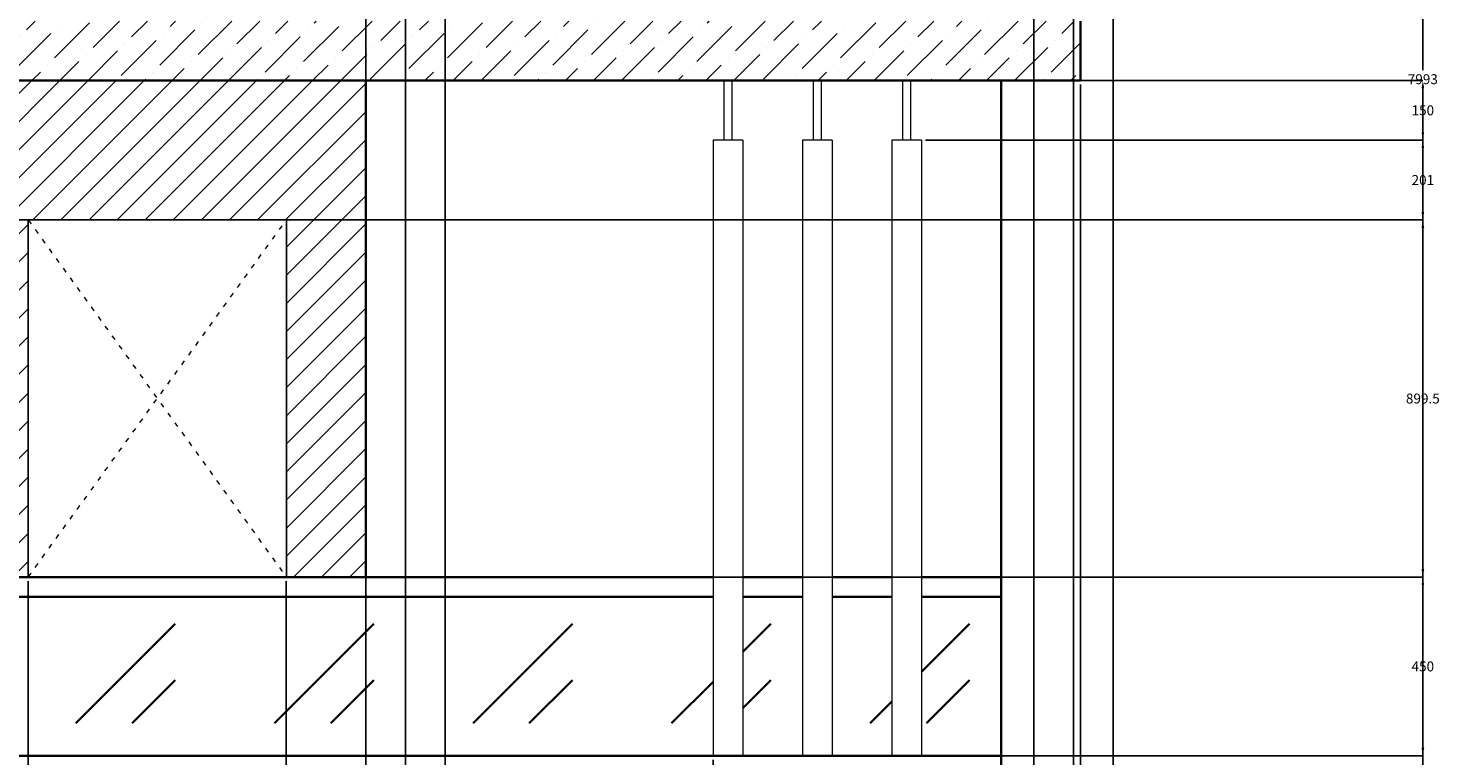
# Model space of a CAD drawing. Units: millimetres. Extents: x -692 to 9639, y -141 to 10345.
# Tile 10 of 19: x 6042 to 9596, y 3148 to 4981. Entities that reach past the tile are written whole.
import ezdxf

# ---------------------------------------------------------------- set-up
doc = ezdxf.new("R2010")
doc.units = ezdxf.units.MM
doc.header["$MEASUREMENT"] = 0
doc.linetypes.add('ACAD_ISO03W100', pattern=[30, 12, -18])
for name, color, linetype, lineweight in [('A-ANNO-DIMS', 2, 'Continuous', 18), ('A-DOOR', 3, 'Continuous', 25), ('A-DOOR-SWNG', 3, 'ACAD_ISO03W100', 18), ('A-ELEV', 7, 'Continuous', 35), ('A-ELEV-DECO', 4, 'Continuous', 18), ('A-ELEV-PATT', 8, 'Continuous', 13)]:
    doc.layers.add(name, color=color, linetype=linetype, lineweight=lineweight)
doc.styles.get("Standard").update_dxf_attribs({"font": 'arial.ttf'})
doc.dimstyles.get("Standard").update_dxf_attribs({"dimtxt": 25, "dimasz": 20, "dimexe": 0.18, "dimexo": 10, "dimgap": 10, "dimtad": 0, "dimtih": 1, "dimtoh": 1, "dimdec": 0, "dimzin": 0, "dimdsep": 46, "dimtxsty": 'Standard', "dimcen": 10, "dimadec": 0, "dimazin": 0, "dimtfac": 1, "dimtdec": 0, "dimtofl": 0, "dimtmove": 0, "dimatfit": 3, "dimfxl": 1, "dimtolj": 1, "dimtzin": 0, "dimarcsym": 0})

# ---------------------------------------------------------------- blocks, each defined once
blk = doc.blocks.new('*D7')
at = {"layer": 'A-ANNO-DIMS', "color": 0, "lineweight": -2, "transparency": 16777216}
for p, q in [((8481.5, 9848.8), (-649.1, 9848.8)), ((-648.9, 9828.8), (-648.9, 5124.9)), ((-648.9, 375.6), (-648.9, 5079.4)), ((2463.7, 355.6), (-649.1, 355.6))]:
    blk.add_line(p, q, dxfattribs=at)
at = {"layer": 'A-ANNO-DIMS', "color": 0, "lineweight": -3, "transparency": 16777216}
for points in [[(-652.2, 9828.8), (-645.6, 9828.8), (-648.9, 9848.8)], [(-652.2, 375.6), (-645.6, 375.6), (-648.9, 355.6)]]:
    blk.add_solid(points, dxfattribs=at)
at = {"layer": 'Defpoints', "color": 0, "lineweight": -3, "transparency": 16777216}
for p in [(-648.9, 9848.8), (8491.5, 9848.8), (2473.7, 355.6)]:
    blk.add_point(p, dxfattribs=at)
at = {"layer": 'A-ANNO-DIMS', "color": 0, "transparency": 16777216, "insert": (-648.9, 5102.2), "char_height": 25, "attachment_point": 5}
blk.add_mtext('\\A1;9493', dxfattribs=at)
blk = doc.blocks.new('*D9')
at = {"layer": 'A-ANNO-DIMS', "color": 0, "lineweight": -2, "transparency": 16777216}
for p, q in [((8501.5, 8848.8), (9553.9, 8848.8)), ((9553.7, 8828.8), (9553.7, 4874.9)), ((9553.7, 875.6), (9553.7, 4829.4)), ((9083.7, 855.6), (9553.9, 855.6))]:
    blk.add_line(p, q, dxfattribs=at)
at = {"layer": 'A-ANNO-DIMS', "color": 0, "lineweight": -3, "transparency": 16777216}
for points in [[(9550.4, 8828.8), (9557.1, 8828.8), (9553.7, 8848.8)], [(9550.4, 875.6), (9557.1, 875.6), (9553.7, 855.6)]]:
    blk.add_solid(points, dxfattribs=at)
at = {"layer": 'Defpoints', "color": 0, "lineweight": -3, "transparency": 16777216}
for p in [(8491.5, 8848.8), (9553.7, 8848.8), (9073.7, 855.6)]:
    blk.add_point(p, dxfattribs=at)
at = {"layer": 'A-ANNO-DIMS', "color": 0, "transparency": 16777216, "insert": (9553.7, 4852.2), "char_height": 25, "attachment_point": 5}
blk.add_mtext('\\A1;7993', dxfattribs=at)
blk = doc.blocks.new('*D32')
at = {"layer": 'A-ANNO-DIMS', "color": 0, "lineweight": -2, "transparency": 16777216}
for p, q in [((6871.7, 10328.8), (6851.7, 10328.8)), ((6891.7, 1865.6), (6891.7, 10329)), ((6991.7, 1765.6), (6991.7, 10329)), ((7011.7, 10328.8), (7031.7, 10328.8))]:
    blk.add_line(p, q, dxfattribs=at)
at = {"layer": 'A-ANNO-DIMS', "color": 0, "lineweight": -3, "transparency": 16777216}
for points in [[(6871.7, 10332.1), (6871.7, 10325.4), (6891.7, 10328.8)], [(7011.7, 10332.1), (7011.7, 10325.4), (6991.7, 10328.8)]]:
    blk.add_solid(points, dxfattribs=at)
at = {"layer": 'Defpoints', "color": 0, "lineweight": -3, "transparency": 16777216}
for p in [(6991.7, 10328.8), (6891.7, 1855.6), (6991.7, 1755.6)]:
    blk.add_point(p, dxfattribs=at)
at = {"layer": 'A-ANNO-DIMS', "color": 0, "transparency": 16777216, "insert": (6941.7, 10328.8), "char_height": 25, "attachment_point": 5}
blk.add_mtext('\\A1;100', dxfattribs=at)
blk = doc.blocks.new('*D33')
at = {"layer": 'A-ANNO-DIMS', "color": 0, "lineweight": -2, "transparency": 16777216}
for p, q in [((6971.7, 10328.8), (6951.7, 10328.8)), ((6991.7, 1765.6), (6991.7, 10329)), ((7091.7, 1665.6), (7091.7, 10329)), ((7111.7, 10328.8), (7131.7, 10328.8))]:
    blk.add_line(p, q, dxfattribs=at)
at = {"layer": 'A-ANNO-DIMS', "color": 0, "lineweight": -3, "transparency": 16777216}
for points in [[(6971.7, 10332.1), (6971.7, 10325.4), (6991.7, 10328.8)], [(7111.7, 10332.1), (7111.7, 10325.4), (7091.7, 10328.8)]]:
    blk.add_solid(points, dxfattribs=at)
at = {"layer": 'Defpoints', "color": 0, "lineweight": -3, "transparency": 16777216}
for p in [(7091.7, 10328.8), (6991.7, 1755.6), (7091.7, 1655.6)]:
    blk.add_point(p, dxfattribs=at)
at = {"layer": 'A-ANNO-DIMS', "color": 0, "transparency": 16777216, "insert": (7041.7, 10328.8), "char_height": 25, "attachment_point": 5}
blk.add_mtext('\\A1;100', dxfattribs=at)
blk = doc.blocks.new('*D34')
at = {"layer": 'A-ANNO-DIMS', "color": 0, "lineweight": -2, "transparency": 16777216}
for p, q in [((7091.7, 1665.6), (7091.7, 10329)), ((7111.7, 10328.8), (7786.7, 10328.8)), ((8553.7, 10328.8), (7878.8, 10328.8)), ((8573.7, 1665.6), (8573.7, 10329))]:
    blk.add_line(p, q, dxfattribs=at)
at = {"layer": 'A-ANNO-DIMS', "color": 0, "lineweight": -3, "transparency": 16777216}
for points in [[(7111.7, 10332.1), (7111.7, 10325.4), (7091.7, 10328.8)], [(8553.7, 10332.1), (8553.7, 10325.4), (8573.7, 10328.8)]]:
    blk.add_solid(points, dxfattribs=at)
at = {"layer": 'Defpoints', "color": 0, "lineweight": -3, "transparency": 16777216}
for p in [(8573.7, 10328.8), (7091.7, 1655.6), (8573.7, 1655.6)]:
    blk.add_point(p, dxfattribs=at)
at = {"layer": 'A-ANNO-DIMS', "color": 0, "transparency": 16777216, "insert": (7832.7, 10328.8), "char_height": 25, "attachment_point": 5}
blk.add_mtext('\\A1;1482', dxfattribs=at)
blk = doc.blocks.new('*D35')
at = {"layer": 'A-ANNO-DIMS', "color": 0, "lineweight": -2, "transparency": 16777216}
for p, q in [((8553.7, 10328.8), (8533.7, 10328.8)), ((8573.7, 1665.6), (8573.7, 10329)), ((8673.7, 1765.6), (8673.7, 10329)), ((8693.7, 10328.8), (8713.7, 10328.8))]:
    blk.add_line(p, q, dxfattribs=at)
at = {"layer": 'A-ANNO-DIMS', "color": 0, "lineweight": -3, "transparency": 16777216}
for points in [[(8553.7, 10332.1), (8553.7, 10325.4), (8573.7, 10328.8)], [(8693.7, 10332.1), (8693.7, 10325.4), (8673.7, 10328.8)]]:
    blk.add_solid(points, dxfattribs=at)
at = {"layer": 'Defpoints', "color": 0, "lineweight": -3, "transparency": 16777216}
for p in [(8673.7, 10328.8), (8673.7, 1755.6), (8573.7, 1655.6)]:
    blk.add_point(p, dxfattribs=at)
at = {"layer": 'A-ANNO-DIMS', "color": 0, "transparency": 16777216, "insert": (8623.7, 10328.8), "char_height": 25, "attachment_point": 5}
blk.add_mtext('\\A1;100', dxfattribs=at)
blk = doc.blocks.new('*D36')
at = {"layer": 'A-ANNO-DIMS', "color": 0, "lineweight": -2, "transparency": 16777216}
for p, q in [((8653.7, 10328.8), (8633.7, 10328.8)), ((8673.7, 1765.6), (8673.7, 10329)), ((8773.7, 1865.6), (8773.7, 10329)), ((8793.7, 10328.8), (8813.7, 10328.8))]:
    blk.add_line(p, q, dxfattribs=at)
at = {"layer": 'A-ANNO-DIMS', "color": 0, "lineweight": -3, "transparency": 16777216}
for points in [[(8653.7, 10332.1), (8653.7, 10325.4), (8673.7, 10328.8)], [(8793.7, 10332.1), (8793.7, 10325.4), (8773.7, 10328.8)]]:
    blk.add_solid(points, dxfattribs=at)
at = {"layer": 'Defpoints', "color": 0, "lineweight": -3, "transparency": 16777216}
for p in [(8773.7, 10328.8), (8773.7, 1855.6), (8673.7, 1755.6)]:
    blk.add_point(p, dxfattribs=at)
at = {"layer": 'A-ANNO-DIMS', "color": 0, "transparency": 16777216, "insert": (8723.7, 10328.8), "char_height": 25, "attachment_point": 5}
blk.add_mtext('\\A1;100', dxfattribs=at)
blk = doc.blocks.new('*D42')
at = {"layer": 'A-ANNO-DIMS', "color": 0, "lineweight": -2, "transparency": 16777216}
for p, q in [((6041.7, 3588.3), (6041.7, -124.6)), ((6691.7, 3588.3), (6691.7, -124.6)), ((6061.7, -124.4), (6329.1, -124.4)), ((6671.7, -124.4), (6404.4, -124.4))]:
    blk.add_line(p, q, dxfattribs=at)
at = {"layer": 'A-ANNO-DIMS', "color": 0, "lineweight": -3, "transparency": 16777216}
for points in [[(6061.7, -121.1), (6061.7, -127.8), (6041.7, -124.4)], [(6671.7, -121.1), (6671.7, -127.8), (6691.7, -124.4)]]:
    blk.add_solid(points, dxfattribs=at)
at = {"layer": 'Defpoints', "color": 0, "lineweight": -3, "transparency": 16777216}
for p in [(6041.7, 3598.3), (6691.7, 3598.3), (6691.7, -124.4)]:
    blk.add_point(p, dxfattribs=at)
at = {"layer": 'A-ANNO-DIMS', "color": 0, "transparency": 16777216, "insert": (6366.7, -124.4), "char_height": 25, "attachment_point": 5}
blk.add_mtext('\\A1;650', dxfattribs=at)
blk = doc.blocks.new('*D43')
at = {"layer": 'A-ANNO-DIMS', "color": 0, "lineweight": -2, "transparency": 16777216}
for p, q in [((6691.7, 3588.3), (6691.7, -124.6)), ((6891.7, 3588.3), (6891.7, -124.6)), ((6711.7, -124.4), (6754, -124.4)), ((6871.7, -124.4), (6829.5, -124.4))]:
    blk.add_line(p, q, dxfattribs=at)
at = {"layer": 'A-ANNO-DIMS', "color": 0, "lineweight": -3, "transparency": 16777216}
for points in [[(6711.7, -121.1), (6711.7, -127.8), (6691.7, -124.4)], [(6871.7, -121.1), (6871.7, -127.8), (6891.7, -124.4)]]:
    blk.add_solid(points, dxfattribs=at)
at = {"layer": 'Defpoints', "color": 0, "lineweight": -3, "transparency": 16777216}
for p in [(6691.7, 3598.3), (6891.7, 3598.3), (6891.7, -124.4)]:
    blk.add_point(p, dxfattribs=at)
at = {"layer": 'A-ANNO-DIMS', "color": 0, "transparency": 16777216, "insert": (6791.7, -124.4), "char_height": 25, "attachment_point": 5}
blk.add_mtext('\\A1;200', dxfattribs=at)
blk = doc.blocks.new('*D44')
at = {"layer": 'A-ANNO-DIMS', "color": 0, "lineweight": -2, "transparency": 16777216}
for p, q in [((6891.7, 3588.3), (6891.7, -124.6)), ((7766.5, 3138.3), (7766.5, -124.6)), ((6911.7, -124.4), (7276.9, -124.4)), ((7746.5, -124.4), (7381.4, -124.4))]:
    blk.add_line(p, q, dxfattribs=at)
at = {"layer": 'A-ANNO-DIMS', "color": 0, "lineweight": -3, "transparency": 16777216}
for points in [[(6911.7, -121.1), (6911.7, -127.8), (6891.7, -124.4)], [(7746.5, -121.1), (7746.5, -127.8), (7766.5, -124.4)]]:
    blk.add_solid(points, dxfattribs=at)
at = {"layer": 'Defpoints', "color": 0, "lineweight": -3, "transparency": 16777216}
for p in [(6891.7, 3598.3), (7766.5, 3148.3), (7766.5, -124.4)]:
    blk.add_point(p, dxfattribs=at)
at = {"layer": 'A-ANNO-DIMS', "color": 0, "transparency": 16777216, "insert": (7329.1, -124.4), "char_height": 25, "attachment_point": 5}
blk.add_mtext('\\A1;874.8', dxfattribs=at)
blk = doc.blocks.new('*D51')
at = {"layer": 'A-ANNO-DIMS', "color": 0, "lineweight": -2, "transparency": 16777216}
for p, q in [((8691.5, 4838.8), (8691.5, -124.6)), ((8491.5, 3138.3), (8491.5, -124.6)), ((8511.5, -124.4), (8553.8, -124.4)), ((8671.5, -124.4), (8629.3, -124.4))]:
    blk.add_line(p, q, dxfattribs=at)
at = {"layer": 'A-ANNO-DIMS', "color": 0, "lineweight": -3, "transparency": 16777216}
for points in [[(8511.5, -121.1), (8511.5, -127.8), (8491.5, -124.4)], [(8671.5, -121.1), (8671.5, -127.8), (8691.5, -124.4)]]:
    blk.add_solid(points, dxfattribs=at)
at = {"layer": 'Defpoints', "color": 0, "lineweight": -3, "transparency": 16777216}
for p in [(8691.5, 4848.8), (8491.5, 3148.3), (8691.5, -124.4)]:
    blk.add_point(p, dxfattribs=at)
at = {"layer": 'A-ANNO-DIMS', "color": 0, "transparency": 16777216, "insert": (8591.5, -124.4), "char_height": 25, "attachment_point": 5}
blk.add_mtext('\\A1;200', dxfattribs=at)
blk = doc.blocks.new('*D71')
at = {"layer": 'A-ANNO-DIMS', "color": 0, "lineweight": -2, "transparency": 16777216}
for p, q in [((5201.5, 3598.3), (9553.9, 3598.3)), ((9553.7, 3578.3), (9553.7, 3396)), ((9553.7, 3168.3), (9553.7, 3350.5)), ((5101.5, 3148.3), (9553.9, 3148.3))]:
    blk.add_line(p, q, dxfattribs=at)
at = {"layer": 'A-ANNO-DIMS', "color": 0, "lineweight": -3, "transparency": 16777216}
for points in [[(9550.4, 3578.3), (9557.1, 3578.3), (9553.7, 3598.3)], [(9550.4, 3168.3), (9557.1, 3168.3), (9553.7, 3148.3)]]:
    blk.add_solid(points, dxfattribs=at)
at = {"layer": 'Defpoints', "color": 0, "lineweight": -3, "transparency": 16777216}
for p in [(5191.5, 3598.3), (9553.7, 3598.3), (5091.5, 3148.3)]:
    blk.add_point(p, dxfattribs=at)
at = {"layer": 'A-ANNO-DIMS', "color": 0, "transparency": 16777216, "insert": (9553.7, 3373.3), "char_height": 25, "attachment_point": 5}
blk.add_mtext('\\A1;450', dxfattribs=at)
blk = doc.blocks.new('*D72')
at = {"layer": 'A-ANNO-DIMS', "color": 0, "lineweight": -2, "transparency": 16777216}
for p, q in [((5201.5, 4497.8), (9553.9, 4497.8)), ((9553.7, 4477.8), (9553.7, 4070.8)), ((9553.7, 3618.3), (9553.7, 4025.3)), ((5201.5, 3598.3), (9553.9, 3598.3))]:
    blk.add_line(p, q, dxfattribs=at)
at = {"layer": 'A-ANNO-DIMS', "color": 0, "lineweight": -3, "transparency": 16777216}
for points in [[(9550.4, 4477.8), (9557.1, 4477.8), (9553.7, 4497.8)], [(9550.4, 3618.3), (9557.1, 3618.3), (9553.7, 3598.3)]]:
    blk.add_solid(points, dxfattribs=at)
at = {"layer": 'Defpoints', "color": 0, "lineweight": -3, "transparency": 16777216}
for p in [(5191.5, 4497.8), (9553.7, 4497.8), (5191.5, 3598.3)]:
    blk.add_point(p, dxfattribs=at)
at = {"layer": 'A-ANNO-DIMS', "color": 0, "transparency": 16777216, "insert": (9553.7, 4048), "char_height": 25, "attachment_point": 5}
blk.add_mtext('\\A1;899.5', dxfattribs=at)
blk = doc.blocks.new('*D73')
at = {"layer": 'A-ANNO-DIMS', "color": 0, "lineweight": -2, "transparency": 16777216}
for p, q in [((8301.5, 4698.8), (9553.9, 4698.8)), ((9553.7, 4678.8), (9553.7, 4621)), ((9553.7, 4517.8), (9553.7, 4575.5)), ((5201.5, 4497.8), (9553.9, 4497.8))]:
    blk.add_line(p, q, dxfattribs=at)
at = {"layer": 'A-ANNO-DIMS', "color": 0, "lineweight": -3, "transparency": 16777216}
for points in [[(9550.4, 4678.8), (9557.1, 4678.8), (9553.7, 4698.8)], [(9550.4, 4517.8), (9557.1, 4517.8), (9553.7, 4497.8)]]:
    blk.add_solid(points, dxfattribs=at)
at = {"layer": 'Defpoints', "color": 0, "lineweight": -3, "transparency": 16777216}
for p in [(8291.5, 4698.8), (9553.7, 4698.8), (5191.5, 4497.8)]:
    blk.add_point(p, dxfattribs=at)
at = {"layer": 'A-ANNO-DIMS', "color": 0, "transparency": 16777216, "insert": (9553.7, 4598.3), "char_height": 25, "attachment_point": 5}
blk.add_mtext('\\A1;201', dxfattribs=at)
blk = doc.blocks.new('*D74')
at = {"layer": 'A-ANNO-DIMS', "color": 0, "lineweight": -2, "transparency": 16777216}
for p, q in [((8274, 4848.8), (9553.9, 4848.8)), ((9553.7, 4828.8), (9553.7, 4796.5)), ((9553.7, 4718.8), (9553.7, 4751)), ((8301.5, 4698.8), (9553.9, 4698.8))]:
    blk.add_line(p, q, dxfattribs=at)
at = {"layer": 'A-ANNO-DIMS', "color": 0, "lineweight": -3, "transparency": 16777216}
for points in [[(9550.4, 4828.8), (9557.1, 4828.8), (9553.7, 4848.8)], [(9550.4, 4718.8), (9557.1, 4718.8), (9553.7, 4698.8)]]:
    blk.add_solid(points, dxfattribs=at)
at = {"layer": 'Defpoints', "color": 0, "lineweight": -3, "transparency": 16777216}
for p in [(8264, 4848.8), (9553.7, 4848.8), (8291.5, 4698.8)]:
    blk.add_point(p, dxfattribs=at)
at = {"layer": 'A-ANNO-DIMS', "color": 0, "transparency": 16777216, "insert": (9553.7, 4773.8), "char_height": 25, "attachment_point": 5}
blk.add_mtext('\\A1;150', dxfattribs=at)

msp = doc.modelspace()

# ---------------------------------------------------------------- hatches: boundary and pattern name
at = {"layer": 'A-ELEV-PATT'}
h = msp.add_hatch(dxfattribs=at)
h.set_pattern_fill('ANSI31', color=256, scale=400)
h.paths.add_polyline_path([(6891.746, 6698.772), (5191.547, 6698.772), (5191.547, 6348.772), (5841.547, 6348.772), (5841.547, 5448.772), (6041.547, 5448.772), (6041.547, 6348.772), (6691.547, 6348.772), (6691.547, 5448.772), (6891.746, 5448.772)])
h.paths.add_polyline_path([(5191.547, 6698.772), (3941.547, 6698.772), (3941.547, 5448.772), (4006.259, 5448.772), (4006.259, 6423.772), (5081.259, 6423.772), (5081.259, 5448.772), (5191.547, 5448.772), (5191.547, 6348.772)])
h.paths.add_polyline_path([(6891.746, 4848.772), (5191.547, 4848.772), (5191.547, 4497.772), (5841.746, 4497.772), (5841.746, 3598.27), (6041.746, 3598.27), (6041.746, 4497.772), (6691.746, 4497.772), (6691.746, 3598.27), (6891.746, 3598.27)])
h.paths.add_polyline_path([(6891.746, 8748.772), (5191.547, 8748.772), (5191.547, 8198.772), (5841.547, 8198.772), (5841.547, 7298.772), (6041.547, 7298.772), (6041.547, 8198.772), (6691.547, 8198.772), (6691.547, 7298.772), (6891.746, 7298.772)])
h = msp.add_hatch(dxfattribs=at)
h.set_pattern_fill('ANSI36', color=256, scale=400)
h.paths.add_polyline_path([(8691.547, 6848.772), (3791.547, 6848.772), (3791.547, 4848.772), (8691.547, 4848.772), (8691.547, 4998.772), (3941.547, 4998.772), (3941.547, 6698.772), (8691.547, 6698.772)])

# ---------------------------------------------------------------- linework, layer by layer
at = {"layer": 'A-DOOR'}
for p, q in [((6041.746, 3598.27), (6041.746, 4497.772)), ((6041.746, 4497.772), (6691.746, 4497.772)), ((6691.746, 3598.27), (6691.746, 4497.772))]:
    msp.add_line(p, q, dxfattribs=at)
at = {"layer": 'A-DOOR-SWNG'}
for p, q in [((6041.746, 3598.27), (6691.946, 4497.772)), ((6041.746, 4497.772), (6691.946, 3598.27))]:
    msp.add_line(p, q, dxfattribs=at)
at = {"layer": 'A-ELEV'}
for p, q in [((8691.547, 4998.772), (8691.547, 4848.772)), ((3791.547, 4848.772), (8691.547, 4848.772)), ((6891.746, 3598.27), (6891.746, 4848.772)), ((8491.547, 4848.772), (8491.547, 1855.575)), ((5191.547, 3598.27), (7766.547, 3598.27)), ((7841.547, 3598.27), (7991.547, 3598.27)), ((8066.547, 3598.27), (8216.547, 3598.27)), ((8291.547, 3598.27), (8491.547, 3598.27)), ((5091.547, 3548.27), (7766.547, 3548.27)), ((7841.547, 3548.27), (7991.547, 3548.27)), ((8066.547, 3548.27), (8216.547, 3548.27)), ((8291.547, 3548.27), (8491.547, 3548.27)), ((6411.99, 3480.203), (6161.99, 3230.203)), ((6911.99, 3480.203), (6661.99, 3230.203)), ((7411.99, 3480.203), (7161.99, 3230.203)), ((7911.99, 3480.203), (7841.547, 3409.759)), ((8411.99, 3480.203), (8291.547, 3359.759)), ((6411.99, 3338.782), (6303.412, 3230.203)), ((6911.99, 3338.782), (6803.412, 3230.203)), ((7411.99, 3338.782), (7303.412, 3230.203)), ((7766.547, 3334.759), (7661.99, 3230.203)), ((7911.99, 3338.782), (7841.547, 3268.338)), ((8411.99, 3338.782), (8303.412, 3230.203)), ((8216.547, 3284.759), (8161.99, 3230.203)), ((5191.547, 3148.27), (8491.547, 3148.27))]:
    msp.add_line(p, q, dxfattribs=at)
at = {"layer": 'A-ELEV-DECO'}
for p, q in [((7794.047, 4698.772), (7794.047, 4848.772)), ((7814.047, 4698.772), (7814.047, 4848.772)), ((8019.047, 4698.772), (8019.047, 4848.772)), ((8039.047, 4698.772), (8039.047, 4848.772)), ((8244.047, 4698.772), (8244.047, 4848.772)), ((8264.047, 4698.772), (8264.047, 4848.772)), ((7766.547, 4698.772), (7766.547, 3148.27)), ((7841.547, 4698.772), (7766.547, 4698.772)), ((7841.547, 4698.772), (7841.547, 3148.27)), ((7991.547, 4698.772), (7991.547, 3148.27)), ((8066.547, 4698.772), (7991.547, 4698.772)), ((8066.547, 4698.772), (8066.547, 3148.27)), ((8216.547, 4698.772), (8216.547, 3148.27)), ((8291.547, 4698.772), (8216.547, 4698.772)), ((8291.547, 4698.772), (8291.547, 3148.27))]:
    msp.add_line(p, q, dxfattribs=at)

# ---------------------------------------------------------------- dimensions: what is measured, and where the dimension line sits
at = {"layer": 'A-ANNO-DIMS'}
for base, p1, p2, override, picture, middle in [((6991.746, 10328.772), (6891.746, 1855.575), (6991.746, 1755.575), {"dimdec": 0, "dimlfac": 1, "dimrnd": 0, "dimzin": 0, "dimdsep": 46, "dimlunit": 2}, '*D32', (6941.746, 10328.772)), ((7091.746, 10328.772), (6991.746, 1755.575), (7091.746, 1655.575), {"dimdec": 0, "dimlfac": 1, "dimrnd": 0, "dimzin": 0, "dimdsep": 46, "dimlunit": 2}, '*D33', (7041.746, 10328.772)), ((8573.746, 10328.772), (7091.746, 1655.575), (8573.746, 1655.575), {"dimdec": 0, "dimlfac": 1, "dimrnd": 0, "dimzin": 0, "dimdsep": 46, "dimlunit": 2}, '*D34', (7832.746, 10328.772)), ((8673.746, 10328.772), (8573.746, 1655.575), (8673.746, 1755.575), {"dimdec": 0, "dimlfac": 1, "dimrnd": 0, "dimzin": 0, "dimdsep": 46, "dimlunit": 2}, '*D35', (8623.746, 10328.772)), ((8773.746, 10328.772), (8673.746, 1755.575), (8773.746, 1855.575), {"dimdec": 0, "dimlfac": 1, "dimrnd": 0, "dimzin": 0, "dimdsep": 46, "dimlunit": 2}, '*D36', (8723.746, 10328.772)), ((8691.547, -124.425), (8491.547, 3148.27), (8691.547, 4848.772), {"dimdec": 0, "dimlfac": 1, "dimrnd": 0, "dimzin": 0, "dimdsep": 46, "dimlunit": 2}, '*D51', (8591.547, -124.425)), ((6691.746, -124.425), (6041.746, 3598.27), (6691.746, 3598.27), {"dimdec": 0, "dimlfac": 1, "dimrnd": 0, "dimzin": 0, "dimdsep": 46, "dimlunit": 2}, '*D42', (6366.746, -124.425)), ((6891.746, -124.425), (6691.746, 3598.27), (6891.746, 3598.27), {"dimdec": 0, "dimlfac": 1, "dimrnd": 0, "dimzin": 0, "dimdsep": 46, "dimlunit": 2}, '*D43', (6791.746, -124.425)), ((7766.547, -124.425), (6891.746, 3598.27), (7766.547, 3148.27), {"dimdec": 1, "dimlfac": 1, "dimrnd": 0, "dimzin": 0, "dimdsep": 46, "dimlunit": 2}, '*D44', (7329.146, -124.425))]:
    dim = msp.add_linear_dim(base=base, p1=p1, p2=p2, dimstyle='Standard', override=override, dxfattribs=at)
    dim.commit()
    dim.dimension.update_dxf_attribs({"geometry": picture, "text_midpoint": middle})
for base, p1, p2, override, picture, middle in [((-648.912, 9848.772), (2473.746, 355.575), (8491.547, 9848.772), {"dimdec": 0, "dimlfac": 1, "dimrnd": 0, "dimzin": 0, "dimdsep": 46, "dimlunit": 2}, '*D7', (-648.912, 5102.173)), ((9553.746, 8848.772), (9073.746, 855.575), (8491.547, 8848.772), {"dimdec": 0, "dimlfac": 1, "dimrnd": 0, "dimzin": 0, "dimdsep": 46, "dimlunit": 2}, '*D9', (9553.746, 4852.173)), ((9553.746, 4848.772), (8291.547, 4698.772), (8264.047, 4848.772), {"dimdec": 0, "dimlfac": 1, "dimrnd": 0, "dimzin": 0, "dimdsep": 46, "dimlunit": 2}, '*D74', (9553.746, 4773.772)), ((9553.746, 4698.772), (5191.547, 4497.772), (8291.547, 4698.772), {"dimdec": 0, "dimlfac": 1, "dimrnd": 0, "dimzin": 0, "dimdsep": 46, "dimlunit": 2}, '*D73', (9553.746, 4598.272)), ((9553.746, 4497.772), (5191.547, 3598.27), (5191.547, 4497.772), {"dimdec": 1, "dimlfac": 1, "dimrnd": 0, "dimzin": 0, "dimdsep": 46, "dimlunit": 2}, '*D72', (9553.746, 4048.021)), ((9553.746, 3598.27), (5091.547, 3148.27), (5191.547, 3598.27), {"dimdec": 0, "dimlfac": 1, "dimrnd": 0, "dimzin": 0, "dimdsep": 46, "dimlunit": 2}, '*D71', (9553.746, 3373.27))]:
    dim = msp.add_linear_dim(base=base, p1=p1, p2=p2, angle=90, dimstyle='Standard', override=override, dxfattribs=at)
    dim.commit()
    dim.dimension.update_dxf_attribs({"geometry": picture, "text_midpoint": middle})

doc.saveas('drawing.dxf')
